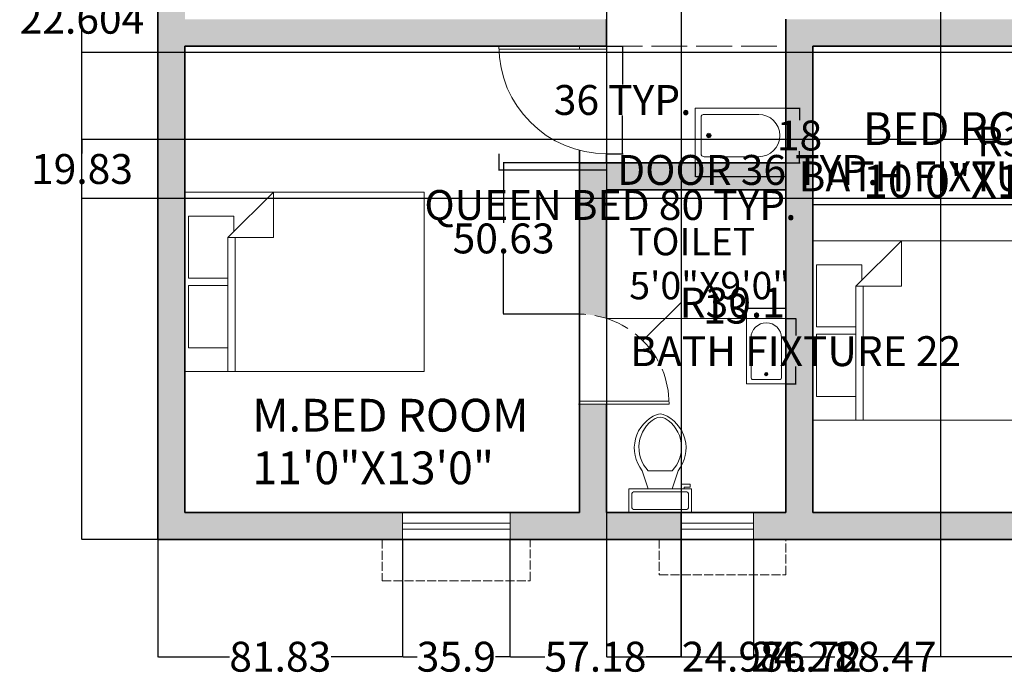
# Model space of a CAD drawing. Units: inches. Extents: x 143 to 746, y -392 to 145.
# Tile 1 of 6: x 143 to 473, y -392 to -173. Entities that reach past the tile are written whole.
import ezdxf

# ---------------------------------------------------------------- set-up
doc = ezdxf.new("R2010")
doc.units = ezdxf.units.IN
doc.header["$MEASUREMENT"] = 0
doc.linetypes.add('ACAD_ISO02W100', pattern=[15, 12, -3])
for name, color, linetype, lineweight in [('A-ANNO-DIMS', 2, 'Continuous', 18), ('A-AREA-IDEN', 7, 'Continuous', 20), ('A-DOOR', 3, 'Continuous', 18), ('A-DOOR-SWNG', 3, 'ACAD_ISO02W100', 13), ('A-FLOR-FIXT', 9, 'Continuous', 18), ('A-FURN', 8, 'Continuous', 18), ('A-GLAZ', 4, 'Continuous', 18), ('A-GLAZ-OVHD', 4, 'ACAD_ISO02W100', 13), ('A-WALL', 7, 'Continuous', 35), ('A-WALL-OVHD', 7, 'ACAD_ISO02W100', 18)]:
    doc.layers.add(name, color=color, linetype=linetype, lineweight=lineweight)
doc.layers.add('A-WALL-PATT', color=252, linetype='Continuous', lineweight=13, true_color=0x939598)
doc.styles.get("Standard").update_dxf_attribs({"font": 'arial.ttf'})
doc.dimstyles.get("Standard").update_dxf_attribs({"dimtxt": 10, "dimasz": 0.18, "dimexe": 0.18, "dimexo": 0.0625, "dimgap": 0.09, "dimtad": 0, "dimtih": 1, "dimtoh": 1, "dimdec": 0, "dimzin": 0, "dimdsep": 46, "dimlunit": 3, "dimtxsty": 'Standard', "dimcen": 0.09, "dimadec": 0, "dimazin": 0, "dimtfac": 1, "dimtdec": 0, "dimtofl": 0, "dimtmove": 0, "dimatfit": 3, "dimfxl": 1, "dimtolj": 1, "dimtzin": 0, "dimarcsym": 0})

# ---------------------------------------------------------------- blocks, each defined once
blk = doc.blocks.new('Toilet - top')
for p, q in [((9.5, -6), (9.5, -2)), ((-10, -8.5), (-8, -8.5)), ((-10, -9.5), (-10, -8.5)), ((-7, -9.5), (-10, -9.5)), ((-8, -8.5), (-8, -8)), ((-7, -8), (-7, -9.5)), ((-4, -8), (-6, -14)), ((4, -8), (6, -14)), ((4, -14), (-4, -14))]:
    blk.add_line(p, q)
blk.add_lwpolyline([(10.5, -8), (10.5, 0), (-10.5, 0), (-10.5, -8)], close=True)
for points in [[(-9.5, -2), (-9.5, -6)], [(8.5, -1), (-8.5, -1)], [(-8.5, -7), (8.5, -7)]]:
    blk.add_lwpolyline(points)
for centre, radius, start, end in [((-8.62, -1.88), 0.884, 81.8699, 188.1301), ((8.62, -1.88), 0.884, 351.8699, 98.1301), ((-8.62, -6.12), 0.884, 171.8699, 278.1301), ((8.62, -6.12), 0.884, 261.8699, 8.1301), ((3.52, -21.58), 12.17, 141.4691, 247.9714), ((4.2, -21.82), 11.33, 136.3677, 238.9468), ((-3.52, -21.58), 12.17, 292.0284, 38.5307), ((-4.2, -21.82), 11.33, 301.053, 43.6321), ((0, -27.88), 4, 245.7318, 294.2682), ((0, -29), 4, 254.8605, 285.1395)]:
    blk.add_arc(centre, radius, start, end)
blk = doc.blocks.new('Bath Tub - 26 x 60 in.')
for p, q in [((8, -18), (10, -18)), ((9, -17), (9, -19))]:
    blk.add_line(p, q)
blk.add_lwpolyline([(0, -36), (0, 0), (60, 0), (60, -36)], close=True)
for points in [[(4, -30), (4, -6)], [(6, -4), (42, -4)], [(42, -32), (6, -32)]]:
    blk.add_lwpolyline(points)
for radius in [1.5, 1]:
    blk.add_circle((9, -18), radius)
for centre, radius, start, end in [((5.75, -5.75), 1.77, 81.8699, 188.1301), ((42, -18), 14, 270, 90), ((5.75, -30.25), 1.77, 171.8699, 278.1301)]:
    blk.add_arc(centre, radius, start, end)
blk = doc.blocks.new('Bed - Queen')
for p, q in [((0, -80.00003), (0, 0)), ((0, 0), (59.99999, 0)), ((59.99999, 0), (59.99999, -80.00003)), ((7.99999, -1.2), (28.79998, -1.2)), ((7.99999, -14.4), (7.99999, -1.2)), ((28.79998, -1.2), (28.79998, -14.4)), ((31.19999, -1.2), (51.99999, -1.2)), ((31.19999, -14.4), (31.19999, -1.2)), ((51.99999, -1.2), (51.99999, -16.4)), ((0, -14.4), (44.8, -14.4)), ((59.99999, -29.6), (44.8, -14.4)), ((44.8, -14.4), (44.8, -29.6)), ((51.99999, -16.4), (46.79936, -16.4)), ((44.8, -16.8), (0, -16.8)), ((44.8, -29.6), (59.99999, -29.6)), ((59.99999, -80.00003), (0, -80.00003))]:
    blk.add_line(p, q)
blk = doc.blocks.new('DOOR-SINGLE-36IN')
for p, q in [((36, 36), (0, 36)), ((36, 35), (0, 35))]:
    blk.add_line(p, q)
blk.add_arc((36, 36), 36, 180, 270)
blk = doc.blocks.new('WINDOW-SHADE-49IN')
at = {"ltscale": 0.25}
for p, q in [((49.48, 13.79), (0, 13.79)), ((0, 13.79), (0, 0)), ((49.48, 0), (49.48, 13.79))]:
    blk.add_line(p, q, dxfattribs=at)
blk = doc.blocks.new('*D10')
at = {"layer": 'A-ANNO-DIMS', "color": 0, "lineweight": -2, "transparency": 16777216}
for p, q in [((399.6, -272.67), (403, -272.67)), ((402.82, -272.85), (402.82, -278.41)), ((402.82, -294.37), (402.82, -288.8)), ((399.6, -294.55), (403, -294.55))]:
    blk.add_line(p, q, dxfattribs=at)
at = {"layer": 'A-ANNO-DIMS', "color": 0, "transparency": 16777216}
for points in [[(402.79, -272.85), (402.85, -272.85), (402.82, -272.67)], [(402.79, -294.37), (402.85, -294.37), (402.82, -294.55)]]:
    blk.add_solid(points, dxfattribs=at)
at = {"layer": 'Defpoints', "color": 0, "transparency": 16777216}
for p in [(399.54, -272.67), (402.82, -272.67), (399.54, -294.55)]:
    blk.add_point(p, dxfattribs=at)
at = {"layer": 'A-ANNO-DIMS', "color": 0, "transparency": 16777216, "insert": (402.82, -283.61), "char_height": 10, "attachment_point": 5}
blk.add_mtext('\\A1;BATH FIXTURE 22', dxfattribs=at)
blk = doc.blocks.new('*D11')
at = {"layer": 'A-ANNO-DIMS', "color": 0, "lineweight": -2, "transparency": 16777216}
for p, q in [((386.41, -269.39), (386.23, -269.39)), ((386.41, -272.6), (386.41, -269.21)), ((399.36, -269.39), (386.59, -269.39)), ((399.54, -272.6), (399.54, -269.21))]:
    blk.add_line(p, q, dxfattribs=at)
at = {"layer": 'A-ANNO-DIMS', "color": 0, "transparency": 16777216}
for points in [[(386.59, -269.36), (386.59, -269.42), (386.41, -269.39)], [(399.36, -269.36), (399.36, -269.42), (399.54, -269.39)]]:
    blk.add_solid(points, dxfattribs=at)
at = {"layer": 'Defpoints', "color": 0, "transparency": 16777216}
for p in [(386.41, -269.39), (386.41, -272.67), (399.54, -272.67)]:
    blk.add_point(p, dxfattribs=at)
at = {"layer": 'A-ANNO-DIMS', "color": 0, "transparency": 16777216, "insert": (379.45, -269.39), "char_height": 10, "attachment_point": 5}
blk.add_mtext('\\A1;13', dxfattribs=at)
blk = doc.blocks.new('*D12')
at = {"layer": 'A-ANNO-DIMS', "color": 0, "lineweight": -2, "transparency": 16777216}
for p, q in [((369.19, -220.67), (369.19, -225.34)), ((399.54, -220.67), (399.54, -225.34)), ((369.37, -225.16), (399.36, -225.16)), ((399.54, -225.16), (399.72, -225.16))]:
    blk.add_line(p, q, dxfattribs=at)
at = {"layer": 'A-ANNO-DIMS', "color": 0, "transparency": 16777216}
for points in [[(369.37, -225.13), (369.37, -225.19), (369.19, -225.16)], [(399.36, -225.13), (399.36, -225.19), (399.54, -225.16)]]:
    blk.add_solid(points, dxfattribs=at)
at = {"layer": 'Defpoints', "color": 0, "transparency": 16777216}
for p in [(369.19, -220.61), (399.54, -220.61), (399.54, -225.16)]:
    blk.add_point(p, dxfattribs=at)
at = {"layer": 'A-ANNO-DIMS', "color": 0, "transparency": 16777216, "insert": (459.12, -225.16), "char_height": 10, "attachment_point": 5}
blk.add_mtext('\\A1;BATH FIXTURE 30', dxfattribs=at)
blk = doc.blocks.new('*D13')
at = {"layer": 'A-ANNO-DIMS', "color": 0, "lineweight": -2, "transparency": 16777216}
for p, q in [((399.6, -202.4), (404.27, -202.4)), ((404.09, -202.58), (404.09, -206.31)), ((404.09, -220.43), (404.09, -216.7)), ((399.6, -220.61), (404.27, -220.61))]:
    blk.add_line(p, q, dxfattribs=at)
at = {"layer": 'A-ANNO-DIMS', "color": 0, "transparency": 16777216}
for points in [[(404.06, -202.58), (404.12, -202.58), (404.09, -202.4)], [(404.06, -220.43), (404.12, -220.43), (404.09, -220.61)]]:
    blk.add_solid(points, dxfattribs=at)
at = {"layer": 'Defpoints', "color": 0, "transparency": 16777216}
for p in [(399.54, -202.4), (404.09, -202.4), (399.54, -220.61)]:
    blk.add_point(p, dxfattribs=at)
at = {"layer": 'A-ANNO-DIMS', "color": 0, "transparency": 16777216, "insert": (404.09, -211.5), "char_height": 10, "attachment_point": 5}
blk.add_mtext('\\A1;18', dxfattribs=at)
blk = doc.blocks.new('*D24')
at = {"layer": 'A-ANNO-DIMS', "color": 0, "lineweight": -2, "transparency": 16777216}
for p, q in [((408.54, -234.73), (408.36, -234.73)), ((408.54, -246.67), (408.54, -234.55)), ((488.36, -234.73), (408.72, -234.73)), ((488.54, -246.67), (488.54, -234.55))]:
    blk.add_line(p, q, dxfattribs=at)
at = {"layer": 'A-ANNO-DIMS', "color": 0, "transparency": 16777216}
for points in [[(408.72, -234.7), (408.72, -234.76), (408.54, -234.73)], [(488.36, -234.7), (488.36, -234.76), (488.54, -234.73)]]:
    blk.add_solid(points, dxfattribs=at)
at = {"layer": 'Defpoints', "color": 0, "transparency": 16777216}
for p in [(408.54, -234.73), (408.54, -246.73), (488.54, -246.73)]:
    blk.add_point(p, dxfattribs=at)
at = {"layer": 'A-ANNO-DIMS', "color": 0, "transparency": 16777216, "insert": (340.86, -234.73), "char_height": 10, "attachment_point": 5}
blk.add_mtext('\\A1;QUEEN BED 80 TYP.', dxfattribs=at)
blk = doc.blocks.new('*D26')
at = {"layer": 'A-ANNO-DIMS', "color": 0, "lineweight": -2, "transparency": 16777216}
for p, q in [((303.54, -217.67), (303.54, -223.19)), ((339.54, -217.67), (339.54, -223.19)), ((303.72, -223.01), (339.36, -223.01)), ((339.54, -223.01), (339.72, -223.01))]:
    blk.add_line(p, q, dxfattribs=at)
at = {"layer": 'A-ANNO-DIMS', "color": 0, "transparency": 16777216}
for points in [[(303.72, -222.98), (303.72, -223.04), (303.54, -223.01)], [(339.36, -222.98), (339.36, -223.04), (339.54, -223.01)]]:
    blk.add_solid(points, dxfattribs=at)
at = {"layer": 'Defpoints', "color": 0, "transparency": 16777216}
for p in [(303.54, -217.61), (339.54, -217.61), (339.54, -223.01)]:
    blk.add_point(p, dxfattribs=at)
at = {"layer": 'A-ANNO-DIMS', "color": 0, "transparency": 16777216, "insert": (386.79, -223.01), "char_height": 10, "attachment_point": 5}
blk.add_mtext('\\A1;DOOR 36 TYP.', dxfattribs=at)
blk = doc.blocks.new('*D27')
at = {"layer": 'A-ANNO-DIMS', "color": 0, "lineweight": -2, "transparency": 16777216}
for p, q in [((339.6, -181.61), (345.12, -181.61)), ((344.94, -181.79), (344.94, -194.41)), ((344.94, -217.43), (344.94, -204.81)), ((339.6, -217.61), (345.12, -217.61))]:
    blk.add_line(p, q, dxfattribs=at)
at = {"layer": 'A-ANNO-DIMS', "color": 0, "transparency": 16777216}
for points in [[(344.91, -181.79), (344.97, -181.79), (344.94, -181.61)], [(344.91, -217.43), (344.97, -217.43), (344.94, -217.61)]]:
    blk.add_solid(points, dxfattribs=at)
at = {"layer": 'Defpoints', "color": 0, "transparency": 16777216}
for p in [(339.54, -181.61), (344.94, -181.61), (339.54, -217.61)]:
    blk.add_point(p, dxfattribs=at)
at = {"layer": 'A-ANNO-DIMS', "color": 0, "transparency": 16777216, "insert": (344.94, -199.61), "char_height": 10, "attachment_point": 5}
blk.add_mtext('\\A1;36 TYP.', dxfattribs=at)
blk = doc.blocks.new('*D34')
at = {"layer": 'A-ANNO-DIMS', "color": 0, "lineweight": -2, "transparency": 16777216}
for p, q in [((189.54, -346.67), (189.54, -385.98)), ((271.37, -346.67), (271.37, -385.98)), ((189.72, -385.8), (213.48, -385.8)), ((271.19, -385.8), (247.42, -385.8))]:
    blk.add_line(p, q, dxfattribs=at)
at = {"layer": 'A-ANNO-DIMS', "color": 0, "transparency": 16777216}
for points in [[(189.72, -385.77), (189.72, -385.83), (189.54, -385.8)], [(271.19, -385.77), (271.19, -385.83), (271.37, -385.8)]]:
    blk.add_solid(points, dxfattribs=at)
at = {"layer": 'Defpoints', "color": 0, "transparency": 16777216}
for p in [(189.54, -346.61), (271.37, -346.61), (271.37, -385.8)]:
    blk.add_point(p, dxfattribs=at)
at = {"layer": 'A-ANNO-DIMS', "color": 0, "transparency": 16777216, "insert": (230.45, -385.8), "char_height": 10, "attachment_point": 5}
blk.add_mtext('\\A1;81.83', dxfattribs=at)
blk = doc.blocks.new('*D35')
at = {"layer": 'A-ANNO-DIMS', "color": 0, "lineweight": -2, "transparency": 16777216}
for p, q in [((271.37, -346.67), (271.37, -385.98)), ((307.27, -346.67), (307.27, -385.98)), ((271.55, -385.8), (276.24, -385.8)), ((307.09, -385.8), (302.41, -385.8))]:
    blk.add_line(p, q, dxfattribs=at)
at = {"layer": 'A-ANNO-DIMS', "color": 0, "transparency": 16777216}
for points in [[(271.55, -385.77), (271.55, -385.83), (271.37, -385.8)], [(307.09, -385.77), (307.09, -385.83), (307.27, -385.8)]]:
    blk.add_solid(points, dxfattribs=at)
at = {"layer": 'Defpoints', "color": 0, "transparency": 16777216}
for p in [(271.37, -346.61), (307.27, -346.61), (307.27, -385.8)]:
    blk.add_point(p, dxfattribs=at)
at = {"layer": 'A-ANNO-DIMS', "color": 0, "transparency": 16777216, "insert": (289.32, -385.8), "char_height": 10, "attachment_point": 5}
blk.add_mtext('\\A1;35.9', dxfattribs=at)
blk = doc.blocks.new('*D36')
at = {"layer": 'A-ANNO-DIMS', "color": 0, "lineweight": -2, "transparency": 16777216}
for p, q in [((307.27, -346.67), (307.27, -385.98)), ((364.45, -346.67), (364.45, -385.98)), ((307.45, -385.8), (318.89, -385.8)), ((364.27, -385.8), (352.83, -385.8))]:
    blk.add_line(p, q, dxfattribs=at)
at = {"layer": 'A-ANNO-DIMS', "color": 0, "transparency": 16777216}
for points in [[(307.45, -385.77), (307.45, -385.83), (307.27, -385.8)], [(364.27, -385.77), (364.27, -385.83), (364.45, -385.8)]]:
    blk.add_solid(points, dxfattribs=at)
at = {"layer": 'Defpoints', "color": 0, "transparency": 16777216}
for p in [(307.27, -346.61), (364.45, -346.61), (364.45, -385.8)]:
    blk.add_point(p, dxfattribs=at)
at = {"layer": 'A-ANNO-DIMS', "color": 0, "transparency": 16777216, "insert": (335.86, -385.8), "char_height": 10, "attachment_point": 5}
blk.add_mtext('\\A1;57.18', dxfattribs=at)
blk = doc.blocks.new('*D37')
at = {"layer": 'A-ANNO-DIMS', "color": 0, "lineweight": -2, "transparency": 16777216}
for p, q in [((364.45, -346.67), (364.45, -385.98)), ((388.66, -346.67), (388.66, -385.98)), ((364.63, -385.8), (388.48, -385.8)), ((388.66, -385.8), (388.84, -385.8))]:
    blk.add_line(p, q, dxfattribs=at)
at = {"layer": 'A-ANNO-DIMS', "color": 0, "transparency": 16777216}
for points in [[(364.63, -385.77), (364.63, -385.83), (364.45, -385.8)], [(388.48, -385.77), (388.48, -385.83), (388.66, -385.8)]]:
    blk.add_solid(points, dxfattribs=at)
at = {"layer": 'Defpoints', "color": 0, "transparency": 16777216}
for p in [(364.45, -346.61), (388.66, -346.61), (388.66, -385.8)]:
    blk.add_point(p, dxfattribs=at)
at = {"layer": 'A-ANNO-DIMS', "color": 0, "transparency": 16777216, "insert": (404.92, -385.8), "char_height": 10, "attachment_point": 5}
blk.add_mtext('\\A1;24.21', dxfattribs=at)
blk = doc.blocks.new('*D38')
at = {"layer": 'A-ANNO-DIMS', "color": 0, "lineweight": -2, "transparency": 16777216}
for p, q in [((388.66, -346.67), (388.66, -385.98)), ((477.13, -346.67), (477.13, -385.98)), ((388.84, -385.8), (415.92, -385.8)), ((476.95, -385.8), (449.86, -385.8))]:
    blk.add_line(p, q, dxfattribs=at)
at = {"layer": 'A-ANNO-DIMS', "color": 0, "transparency": 16777216}
for points in [[(388.84, -385.77), (388.84, -385.83), (388.66, -385.8)], [(476.95, -385.77), (476.95, -385.83), (477.13, -385.8)]]:
    blk.add_solid(points, dxfattribs=at)
at = {"layer": 'Defpoints', "color": 0, "transparency": 16777216}
for p in [(388.66, -346.61), (477.13, -346.61), (477.13, -385.8)]:
    blk.add_point(p, dxfattribs=at)
at = {"layer": 'A-ANNO-DIMS', "color": 0, "transparency": 16777216, "insert": (432.89, -385.8), "char_height": 10, "attachment_point": 5}
blk.add_mtext('\\A1;88.47', dxfattribs=at)
blk = doc.blocks.new('*D45')
at = {"layer": 'A-ANNO-DIMS', "color": 0, "lineweight": -2, "transparency": 16777216}
for p, q in [((330.48, 113.48), (163.96, 113.48)), ((164.14, 113.3), (164.14, -111.37)), ((164.14, -346.43), (164.14, -121.76)), ((189.48, -346.61), (163.96, -346.61))]:
    blk.add_line(p, q, dxfattribs=at)
at = {"layer": 'A-ANNO-DIMS', "color": 0, "transparency": 16777216}
for points in [[(164.11, 113.3), (164.17, 113.3), (164.14, 113.48)], [(164.11, -346.43), (164.17, -346.43), (164.14, -346.61)]]:
    blk.add_solid(points, dxfattribs=at)
at = {"layer": 'Defpoints', "color": 0, "transparency": 16777216}
for p in [(164.14, 113.48), (330.54, 113.48), (189.54, -346.61)]:
    blk.add_point(p, dxfattribs=at)
at = {"layer": 'A-ANNO-DIMS', "color": 0, "transparency": 16777216, "insert": (164.14, -116.56), "char_height": 10, "attachment_point": 5}
blk.add_mtext('\\A1;460.1', dxfattribs=at)
blk = doc.blocks.new('*D51')
at = {"layer": 'A-ANNO-DIMS', "color": 0, "lineweight": -2, "transparency": 16777216}
for p, q in [((339.54, -2.09), (339.54, -385.98)), ((364.51, -2.09), (364.51, -385.98)), ((339.72, -385.8), (364.33, -385.8)), ((364.51, -385.8), (364.69, -385.8))]:
    blk.add_line(p, q, dxfattribs=at)
at = {"layer": 'A-ANNO-DIMS', "color": 0, "transparency": 16777216}
for points in [[(339.72, -385.77), (339.72, -385.83), (339.54, -385.8)], [(364.33, -385.77), (364.33, -385.83), (364.51, -385.8)]]:
    blk.add_solid(points, dxfattribs=at)
at = {"layer": 'Defpoints', "color": 0, "transparency": 16777216}
for p in [(339.54, -2.03), (364.51, -2.03), (364.51, -385.8)]:
    blk.add_point(p, dxfattribs=at)
at = {"layer": 'A-ANNO-DIMS', "color": 0, "transparency": 16777216, "insert": (381.74, -385.8), "char_height": 10, "attachment_point": 5}
blk.add_mtext('\\A1;24.97', dxfattribs=at)
blk = doc.blocks.new('*D52')
at = {"layer": 'A-ANNO-DIMS', "color": 0, "lineweight": -2, "transparency": 16777216}
for p, q in [((364.51, -2.09), (364.51, -385.98)), ((451.23, -2.09), (451.23, -385.98)), ((364.69, -385.8), (390.95, -385.8)), ((451.05, -385.8), (424.79, -385.8))]:
    blk.add_line(p, q, dxfattribs=at)
at = {"layer": 'A-ANNO-DIMS', "color": 0, "transparency": 16777216}
for points in [[(364.69, -385.77), (364.69, -385.83), (364.51, -385.8)], [(451.05, -385.77), (451.05, -385.83), (451.23, -385.8)]]:
    blk.add_solid(points, dxfattribs=at)
at = {"layer": 'Defpoints', "color": 0, "transparency": 16777216}
for p in [(364.51, -2.03), (451.23, -2.03), (451.23, -385.8)]:
    blk.add_point(p, dxfattribs=at)
at = {"layer": 'A-ANNO-DIMS', "color": 0, "transparency": 16777216, "insert": (407.87, -385.8), "char_height": 10, "attachment_point": 5}
blk.add_mtext('\\A1;86.72', dxfattribs=at)
blk = doc.blocks.new('*D66')
at = {"layer": 'A-ANNO-DIMS', "color": 0, "lineweight": -2, "transparency": 16777216}
for p, q in [((537.48, -212.78), (163.96, -212.78)), ((164.14, -212.96), (164.14, -217.49)), ((164.14, -232.43), (164.14, -227.89)), ((537.48, -232.61), (163.96, -232.61))]:
    blk.add_line(p, q, dxfattribs=at)
at = {"layer": 'A-ANNO-DIMS', "color": 0, "transparency": 16777216}
for points in [[(164.11, -212.96), (164.17, -212.96), (164.14, -212.78)], [(164.11, -232.43), (164.17, -232.43), (164.14, -232.61)]]:
    blk.add_solid(points, dxfattribs=at)
at = {"layer": 'Defpoints', "color": 0, "transparency": 16777216}
for p in [(537.54, -212.78), (164.14, -232.61), (537.54, -232.61)]:
    blk.add_point(p, dxfattribs=at)
at = {"layer": 'A-ANNO-DIMS', "color": 0, "transparency": 16777216, "insert": (164.14, -222.69), "char_height": 10, "attachment_point": 5}
blk.add_mtext('\\A1;19.83', dxfattribs=at)
blk = doc.blocks.new('*D70')
at = {"layer": 'A-ANNO-DIMS', "color": 0, "lineweight": -2, "transparency": 16777216}
for p, q in [((645.96, -161.14), (163.96, -161.14)), ((164.14, -161.32), (164.14, -167.24)), ((164.14, -183.56), (164.14, -177.64)), ((645.96, -183.74), (163.96, -183.74))]:
    blk.add_line(p, q, dxfattribs=at)
at = {"layer": 'A-ANNO-DIMS', "color": 0, "transparency": 16777216}
for points in [[(164.11, -161.32), (164.17, -161.32), (164.14, -161.14)], [(164.11, -183.56), (164.17, -183.56), (164.14, -183.74)]]:
    blk.add_solid(points, dxfattribs=at)
at = {"layer": 'Defpoints', "color": 0, "transparency": 16777216}
for p in [(646.02, -161.14), (164.14, -183.74), (646.02, -183.74)]:
    blk.add_point(p, dxfattribs=at)
at = {"layer": 'A-ANNO-DIMS', "color": 0, "transparency": 16777216, "insert": (164.14, -172.44), "char_height": 10, "attachment_point": 5}
blk.add_mtext('\\A1;22.604', dxfattribs=at)
blk = doc.blocks.new('*D72')
at = {"layer": 'A-ANNO-DIMS', "color": 0, "lineweight": -2, "transparency": 16777216}
for p, q in [((330.48, -220.61), (304.96, -220.61)), ((305.14, -220.79), (305.14, -240.72)), ((305.14, -271.06), (305.14, -251.12)), ((330.48, -271.24), (304.96, -271.24))]:
    blk.add_line(p, q, dxfattribs=at)
at = {"layer": 'A-ANNO-DIMS', "color": 0, "transparency": 16777216}
for points in [[(305.11, -220.79), (305.17, -220.79), (305.14, -220.61)], [(305.11, -271.06), (305.17, -271.06), (305.14, -271.24)]]:
    blk.add_solid(points, dxfattribs=at)
at = {"layer": 'Defpoints', "color": 0, "transparency": 16777216}
for p in [(305.14, -220.61), (330.54, -220.61), (330.54, -271.24)]:
    blk.add_point(p, dxfattribs=at)
at = {"layer": 'A-ANNO-DIMS', "color": 0, "transparency": 16777216, "insert": (305.14, -245.92), "char_height": 10, "attachment_point": 5}
blk.add_mtext('\\A1;50.63', dxfattribs=at)
blk = doc.blocks.new('*D77')
at = {"layer": 'A-ANNO-DIMS', "color": 0, "lineweight": -2, "transparency": 16777216}
for p, q in [((528.45, -173), (528.63, -173)), ((528.54, -173.09), (528.54, -172.91)), ((487.58, -213.51), (502.81, -198.45)), ((487.4, -213.51), (487.58, -213.51))]:
    blk.add_line(p, q, dxfattribs=at)
at = {"layer": 'A-ANNO-DIMS', "color": 0, "transparency": 16777216}
blk.add_solid([(502.79, -198.43), (502.83, -198.47), (502.94, -198.32)], dxfattribs=at)
at = {"layer": 'Defpoints', "color": 0, "transparency": 16777216}
for p in [(528.54, -173), (502.94, -198.32)]:
    blk.add_point(p, dxfattribs=at)
at = {"layer": 'A-ANNO-DIMS', "color": 0, "transparency": 16777216, "insert": (475.37, -213.51), "char_height": 10, "attachment_point": 5}
blk.add_mtext('\\A1;R36', dxfattribs=at)
blk = doc.blocks.new('*D78')
at = {"layer": 'A-ANNO-DIMS', "color": 0, "lineweight": -2, "transparency": 16777216}
for p, q in [((364.52, -267.38), (351.84, -279.98)), ((364.7, -267.38), (364.52, -267.38)), ((330.28, -301.34), (330.46, -301.34)), ((330.37, -301.43), (330.37, -301.25))]:
    blk.add_line(p, q, dxfattribs=at)
at = {"layer": 'A-ANNO-DIMS', "color": 0, "transparency": 16777216}
blk.add_solid([(351.82, -279.96), (351.86, -280.01), (351.72, -280.11)], dxfattribs=at)
at = {"layer": 'Defpoints', "color": 0, "transparency": 16777216}
for p in [(351.72, -280.11), (330.37, -301.34)]:
    blk.add_point(p, dxfattribs=at)
at = {"layer": 'A-ANNO-DIMS', "color": 0, "transparency": 16777216, "insert": (381.6, -267.38), "char_height": 10, "attachment_point": 5}
blk.add_mtext('\\A1;R30.1', dxfattribs=at)

msp = doc.modelspace()

# ---------------------------------------------------------------- hatches: boundary and pattern name
at = {"layer": 'A-WALL-PATT'}
h = msp.add_hatch(color=256, dxfattribs=at)
h.dxf.hatch_style = 1
h.paths.add_polyline_path([(198.538, 19.3924), (257.4275, 19.3924), (257.4275, 28.3924), (189.538, 28.3924), (189.538, -95.6731, -0.06325422), (198.538, -96.8162)])
h.paths.add_polyline_path([(339.538, 66.969), (471.538, 66.969), (472.538, 66.969), (472.538, 31.3924), (472.538, 6.969), (451.2296, 6.969), (451.2296, -2.031), (472.538, -2.031), (472.538, -82.6076), (544.538, -82.6076), (544.538, -38.6894), (535.538, -38.6894), (535.538, -73.6076), (481.538, -73.6076), (481.538, 22.3924), (498.7149, 22.3924), (498.7149, 31.3924), (481.538, 31.3924), (481.538, 66.969), (481.538, 113.4779), (471.538, 113.4779), (471.538, 75.969), (339.538, 75.969), (339.538, 113.4779), (330.538, 113.4779), (330.538, 66.969), (330.538, 28.3924), (293.6446, 28.3924), (293.6446, 19.3924), (330.538, 19.3924), (330.538, 6.969), (330.538, -2.031), (364.5099, -2.031), (364.5099, 6.969), (339.538, 6.969)])
h.paths.add_polyline_path([(570.63, 31.3924), (544.538, 31.3924), (524.7988, 31.3924), (524.7988, 22.3924), (535.538, 22.3924), (535.538, -9.9696, -0.0761882), (544.538, -8.6878), (544.538, 22.3924), (570.63, 22.3924)])
h.paths.add_polyline_path([(679.538, 31.3924), (618.768, 31.3924), (618.768, 22.3924), (670.538, 22.3924), (670.538, -54.5218), (679.538, -54.5218)])
h.paths.add_polyline_path([(679.538, -90.0753), (670.538, -90.0753), (670.538, -121.6076), (537.538, -121.6076), (528.538, -121.6076), (528.538, -130.6076), (537.538, -130.6076), (670.538, -130.6076), (670.538, -150.8923), (679.538, -150.8923)])
h.paths.add_polyline_path([(679.538, -187.0502), (670.538, -187.0502), (670.538, -232.6076), (636.538, -232.6076, -0.07632083), (635.1562, -241.6076), (670.538, -241.6076), (670.538, -256.599), (679.538, -256.599)])
h.paths.add_polyline_path([(606.538, -232.6076), (537.538, -232.6076), (537.538, -241.6076), (597.538, -241.6076), (597.538, -337.6076), (590.545, -337.6076), (590.545, -346.6076), (679.538, -346.6076), (679.538, -316.1251), (670.538, -316.1251), (670.538, -337.6076), (606.538, -337.6076)])
h.paths.add_polyline_path([(537.538, -181.6076), (537.538, -172.6076), (528.538, -172.6076), (528.538, -209.005), (528.538, -269.6672, -0.07632083), (537.538, -271.0491)])
h.paths.add_polyline_path([(566.8252, -337.6076), (537.538, -337.6076), (537.538, -299.6672), (528.538, -299.6672), (528.538, -337.6076), (513.484, -337.6076), (513.484, -346.6076), (566.8252, -346.6076)])
h.paths.add_polyline_path([(477.1278, -337.6076), (408.538, -337.6076), (408.538, -229.6076), (408.538, -181.6076), (493.5793, -181.6076, -0.06316411), (492.538, -172.6076), (399.538, -172.6076), (399.538, -229.6076), (399.538, -337.6076), (388.659, -337.6076), (388.659, -346.6076), (477.1278, -346.6076)])
h.paths.add_polyline_path([(364.4504, -337.6076), (339.538, -337.6076), (339.538, -301.3371), (330.538, -301.3371), (330.538, -337.6076), (307.2736, -337.6076), (307.2736, -346.6076), (364.4504, -346.6076)])
h.paths.add_polyline_path([(339.538, -229.6076), (399.538, -229.6076), (399.538, -220.6076), (369.1898, -220.6076), (330.538, -220.6076), (330.538, -271.2389, -0.07612824), (339.538, -272.6672)])
h.paths.add_polyline_path([(271.3704, -337.6076), (198.538, -337.6076), (198.538, -181.6076), (339.538, -181.6076), (339.538, -172.6076), (198.538, -172.6076), (198.538, -131.6731), (189.538, -131.6731), (189.538, -346.6076), (271.3704, -346.6076)])

# ---------------------------------------------------------------- linework, layer by layer
at = {"layer": 'A-DOOR'}
for p, q in [((330.538, -182.6076), (330.538, -181.6076)), ((339.538, -181.6076), (339.538, -182.6076)), ((339.538, -182.6076), (339.538, -181.6076)), ((330.538, -301.3371), (330.538, -271.2389)), ((330.538, -300.3371), (360.4735, -300.3371)), ((330.538, -301.3371), (360.4735, -301.3371))]:
    msp.add_line(p, q, dxfattribs=at)
at = {"layer": 'A-DOOR-SWNG'}
msp.add_arc((330.3748, -301.3371), 30.0987, 0, 89.689278, dxfattribs=at)
at = {"layer": 'A-FLOR-FIXT'}
msp.add_line((339.538, -272.6672), (399.538, -272.6672), dxfattribs=at)
at = {"layer": 'A-GLAZ'}
for p, q in [((271.3704, -342.1076), (271.3704, -337.6076)), ((271.3704, -337.6076), (271.3704, -346.6076)), ((307.2736, -337.6076), (307.2736, -346.6076)), ((364.4504, -342.1076), (364.4504, -337.6076)), ((364.4504, -337.6076), (364.4504, -346.6076)), ((388.659, -337.6076), (388.659, -346.6076)), ((307.2736, -341.1076), (271.3704, -341.1076)), ((388.659, -341.1076), (364.4504, -341.1076)), ((307.2736, -343.1076), (271.3704, -343.1076)), ((388.659, -343.1076), (364.4504, -343.1076))]:
    msp.add_line(p, q, dxfattribs=at)
at = {"layer": 'A-GLAZ-OVHD', "ltscale": 0.25}
for p, q in [((357.1927, -346.6076), (357.1927, -358.4113)), ((399.553, -358.4113), (399.553, -346.6076)), ((357.1927, -358.4113), (399.553, -358.4113))]:
    msp.add_line(p, q, dxfattribs=at)
at = {"layer": 'A-WALL'}
for p, q in [((189.538, 28.3924), (189.538, -346.6076)), ((339.538, -181.6076), (339.538, -172.6076)), ((399.538, -172.6076), (399.538, -229.6076)), ((198.538, -181.6076), (339.538, -181.6076)), ((198.538, -181.6076), (198.538, -337.6076)), ((493.5793, -181.6076), (408.538, -181.6076)), ((408.538, -181.6076), (408.538, -229.6076)), ((330.538, -337.6076), (330.538, -216.4644)), ((339.538, -220.6076), (339.538, -217.6076)), ((399.538, -220.6076), (330.538, -220.6076)), ((399.538, -229.6076), (339.538, -229.6076)), ((339.538, -272.6672), (339.538, -229.6076)), ((399.538, -337.6076), (399.538, -229.6076)), ((408.538, -337.6076), (408.538, -229.6076)), ((339.538, -337.6076), (339.538, -301.3371)), ((198.538, -337.6076), (330.538, -337.6076)), ((339.538, -337.6076), (399.538, -337.6076)), ((408.538, -337.6076), (528.538, -337.6076)), ((189.538, -346.6076), (679.538, -346.6076)), ((198.538, -346.6076), (330.538, -346.6076)), ((339.538, -346.6076), (399.538, -346.6076)), ((408.538, -346.6076), (528.538, -346.6076))]:
    msp.add_line(p, q, dxfattribs=at)
at = {"layer": 'A-WALL-OVHD'}
msp.add_line((339.538, -181.6076), (399.538, -181.6076), dxfattribs=at)

# ---------------------------------------------------------------- block references
at = {"layer": 'A-DOOR'}
msp.add_blockref('DOOR-SINGLE-36IN', (303.538, -217.608), dxfattribs=at)
at = {"layer": 'A-FLOR-FIXT', "xscale": 0.5058036704762096, "yscale": 0.5058036704762096, "zscale": 0.5058036704762096}
msp.add_blockref('Bath Tub - 26 x 60 in.', (369.1898, -202.3987), dxfattribs=at)
at = {"layer": 'A-FLOR-FIXT', "xscale": 0.3646808545639447, "yscale": 0.3646808545639447, "zscale": 0.3646808545639447, "rotation": 90}
msp.add_blockref('Bath Tub - 26 x 60 in.', (386.4095, -294.548), dxfattribs=at)
at = {"layer": 'A-FLOR-FIXT', "rotation": 180}
msp.add_blockref('Toilet - top', (357.4935, -337.6076), dxfattribs=at)
at = {"layer": 'A-FURN', "rotation": 90}
for p in [(198.538, -290.4584), (408.538, -306.7314)]:
    msp.add_blockref('Bed - Queen', p, dxfattribs=at)
at = {"layer": 'A-GLAZ-OVHD', "rotation": 180}
msp.add_blockref('WINDOW-SHADE-49IN', (314.017, -346.6072), dxfattribs=at)

# ---------------------------------------------------------------- texts
at = {"layer": 'A-AREA-IDEN'}
for s, height, p in [('BED ROOM', 10.95807, (425.3066, -214.6495)), ('10\'0"X13\'0"', 10.958074, (425.3066, -232.2526)), ('TOILET', 9.17063, (347.1579, -251.5421)), ('5\'0"X9\'0"', 9.17063, (347.1579, -266.2739)), ('M.BED ROOM', 10.95807, (221.0914, -310.5145)), ('11\'0"X13\'0"', 10.958074, (221.0914, -328.1177))]:
    msp.add_text(s, height=height, dxfattribs=at).set_placement(p)

# ---------------------------------------------------------------- dimensions: what is measured, and where the dimension line sits
at = {"layer": 'A-ANNO-DIMS'}
for base, p1, p2, angle, override, picture, middle in [((164.138, 113.4779), (189.538, -346.6076), (330.538, 113.4779), 90, {"dimdec": 1, "dimlfac": 1, "dimrnd": 0, "dimzin": 0, "dimdsep": 46, "dimlunit": 2}, '*D45', (164.138, -116.5649)), ((164.138, -183.7414), (646.0181, -161.1374), (646.0181, -183.7414), 90, {"dimdec": 3, "dimlfac": 1, "dimrnd": 0, "dimzin": 0, "dimdsep": 46, "dimlunit": 2}, '*D70', (164.138, -172.4394)), ((404.0903, -202.3987), (399.538, -220.6076), (399.538, -202.3987), 90, {"dimdec": 0, "dimlfac": 1, "dimrnd": 0, "dimzin": 0, "dimdsep": 46, "dimlunit": 2}, '*D13', (404.0903, -211.5031)), ((164.138, -232.6076), (537.538, -212.7788), (537.538, -232.6076), 90, {"dimdec": 2, "dimlfac": 1, "dimrnd": 0, "dimzin": 0, "dimdsep": 46, "dimlunit": 2}, '*D66', (164.138, -222.6932)), ((305.138, -220.6076), (330.538, -271.2389), (330.538, -220.6076), 90, {"dimdec": 2, "dimlfac": 1, "dimrnd": 0, "dimzin": 0, "dimdsep": 46, "dimlunit": 2}, '*D72', (305.138, -245.9232)), ((386.4095, -269.385), (399.538, -272.6672), (386.4095, -272.6672), 180, {"dimdec": 0, "dimlfac": 1, "dimrnd": 0, "dimzin": 0, "dimdsep": 46, "dimlunit": 2}, '*D11', (379.4478, -269.385))]:
    dim = msp.add_linear_dim(base=base, p1=p1, p2=p2, angle=angle, dimstyle='Standard', override=override, dxfattribs=at)
    dim.commit()
    dim.dimension.update_dxf_attribs({"geometry": picture, "text_midpoint": middle})
for base, p1, p2, override, picture, middle in [((364.5099, -385.7951), (339.538, -2.031), (364.5099, -2.031), {"dimdec": 2, "dimlfac": 1, "dimrnd": 0, "dimzin": 0, "dimdsep": 46, "dimlunit": 2}, '*D51', (381.7376, -385.7951)), ((451.2296, -385.7951), (364.5099, -2.031), (451.2296, -2.031), {"dimdec": 2, "dimlfac": 1, "dimrnd": 0, "dimzin": 0, "dimdsep": 46, "dimlunit": 2}, '*D52', (407.8698, -385.7951)), ((271.3704, -385.7951), (189.538, -346.6076), (271.3704, -346.6076), {"dimdec": 2, "dimlfac": 1, "dimrnd": 0, "dimzin": 0, "dimdsep": 46, "dimlunit": 2}, '*D34', (230.4542, -385.7951)), ((307.2736, -385.7951), (271.3704, -346.6076), (307.2736, -346.6076), {"dimdec": 1, "dimlfac": 1, "dimrnd": 0, "dimzin": 0, "dimdsep": 46, "dimlunit": 2}, '*D35', (289.322, -385.7951)), ((364.4504, -385.7951), (307.2736, -346.6076), (364.4504, -346.6076), {"dimdec": 2, "dimlfac": 1, "dimrnd": 0, "dimzin": 0, "dimdsep": 46, "dimlunit": 2}, '*D36', (335.862, -385.7951)), ((388.659, -385.7951), (364.4504, -346.6076), (388.659, -346.6076), {"dimdec": 2, "dimlfac": 1, "dimrnd": 0, "dimzin": 0, "dimdsep": 46, "dimlunit": 2}, '*D37', (404.9215, -385.7951)), ((477.1278, -385.7951), (388.659, -346.6076), (477.1278, -346.6076), {"dimdec": 2, "dimlfac": 1, "dimrnd": 0, "dimzin": 0, "dimdsep": 46, "dimlunit": 2}, '*D38', (432.8934, -385.7951))]:
    dim = msp.add_linear_dim(base=base, p1=p1, p2=p2, dimstyle='Standard', override=override, dxfattribs=at)
    dim.commit()
    dim.dimension.update_dxf_attribs({"geometry": picture, "text_midpoint": middle})
for center, mpoint, override, picture, middle in [((528.538, -173.0028), (502.9411, -198.3199), {"dimdec": 0, "dimlfac": 1, "dimrnd": 0, "dimzin": 0, "dimdsep": 46, "dimlunit": 2}, '*D77', (475.3689, -213.5101)), ((330.3748, -301.3371), (351.7152, -280.1118), {"dimdec": 1, "dimlfac": 1, "dimrnd": 0, "dimzin": 0, "dimdsep": 46, "dimlunit": 2}, '*D78', (381.5972, -267.3765))]:
    dim = msp.add_radius_dim(center=center, mpoint=mpoint, dimstyle='Standard', override=override, dxfattribs=at)
    dim.commit()
    dim.dimension.update_dxf_attribs({"geometry": picture, "text_midpoint": middle, "dimtype": 164})
for base, p1, p2, angle, text, picture, middle in [((344.938, -181.6076), (339.538, -217.6076), (339.538, -181.6076), 90, '<> TYP.', '*D27', (344.938, -199.6076)), ((408.538, -234.7314), (488.5381, -246.7314), (408.538, -246.7314), 180, 'QUEEN BED <> TYP.', '*D24', (340.8567, -234.7314)), ((402.8202, -272.6672), (399.538, -294.548), (399.538, -272.6672), 90, 'BATH FIXTURE <>', '*D10', (402.8202, -283.6076))]:
    dim = msp.add_linear_dim(base=base, p1=p1, p2=p2, angle=angle, text=text, dimstyle='Standard', override={"dimdec": 0, "dimlfac": 1, "dimrnd": 0, "dimzin": 0, "dimdsep": 46, "dimlunit": 2}, dxfattribs=at)
    dim.commit()
    dim.dimension.update_dxf_attribs({"geometry": picture, "text_midpoint": middle})
for base, p1, p2, text, picture, middle in [((339.538, -223.0076), (303.538, -217.6076), (339.538, -217.6076), 'DOOR <> TYP.', '*D26', (386.793, -223.0076)), ((399.538, -225.1598), (369.1898, -220.6076), (399.538, -220.6076), 'BATH FIXTURE <>', '*D12', (459.1225, -225.1598))]:
    dim = msp.add_linear_dim(base=base, p1=p1, p2=p2, text=text, dimstyle='Standard', override={"dimdec": 0, "dimlfac": 1, "dimrnd": 0, "dimzin": 0, "dimdsep": 46, "dimlunit": 2}, dxfattribs=at)
    dim.commit()
    dim.dimension.update_dxf_attribs({"geometry": picture, "text_midpoint": middle})

doc.saveas('drawing.dxf')
